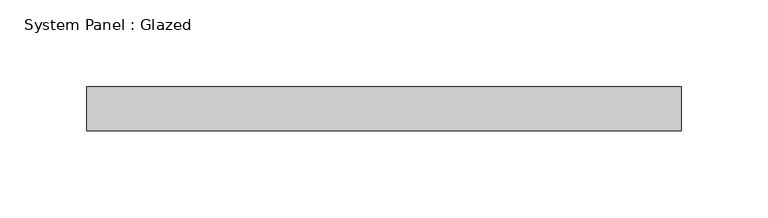
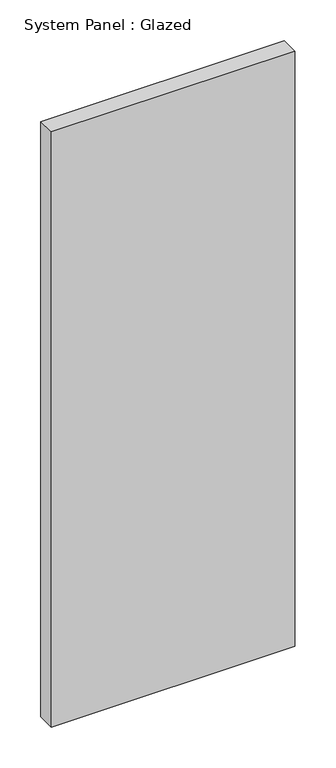
"""IFC4 building model written with IfcOpenShell, lengths in millimetres: plate geometry, System Panel : Glazed."""

from ifc_helpers import new_model, si_unit, origin, origin_with_axes, place, context, project, spatial, polyline, outline, extrude, source, transform, mapped, element, save


def system_panel_glazed_48942baa(model_context):
    return source(origin(), model_context, "Body", "SweptSolid", [
        extrude(outline(polyline([(171.45, 19.05), (-171.45, 19.05), (-171.45, 44.45), (171.45, 44.45), (171.45, 19.05)])), origin_with_axes(), (0.0, 0.0, 1.0), 886.8833333),
    ])


if __name__ == "__main__":
    model = new_model("IFC4")
    model_context = context("Model", 3, world=origin())
    ifc_project = project(units=[si_unit("LENGTHUNIT", "METRE", prefix="MILLI")], contexts=[model_context])
    site = spatial("IfcSite", under=ifc_project)
    building = spatial("IfcBuilding", under=site)
    placement = place(None, origin())
    system_panel_glazed_shape = system_panel_glazed_48942baa(model_context)
    element("IfcPlate", 1, ObjectType="System Panel : Glazed", at=placement, inside=building, context=model_context, shape_type="MappedRepresentation", body=[
        mapped(system_panel_glazed_shape, transform((0.0, 0.0, 0.0), x_axis=(1.0, 0.0, 0.0), y_axis=(0.0, 1.0, 0.0), z_axis=(0.0, 0.0, 1.0))),
    ])
    save(model, "model.ifc")

# Revit data of these elements
# Type "System Panel : Glazed"
#   Construction Type Id = "GSP4R"
#   Analytic Construction = "1/8 in Pilkington single glazing"
#   Visual Light Transmittance = 0.9
#   Solar Heat Gain Coefficient = 0.86
#   Heat Transfer Coefficient (U) = 1.18115 BTU/(h·ft²·°F)
# Element 1 (IfcPlate, "System Panel : Glazed")
#   Materials on its faces: "Glass"
# Materials
#   "Glass": class "Glass", colour RGB 0 128 192, transparency 0.75, Description = "Soda Lime Glass", Cost = 0
